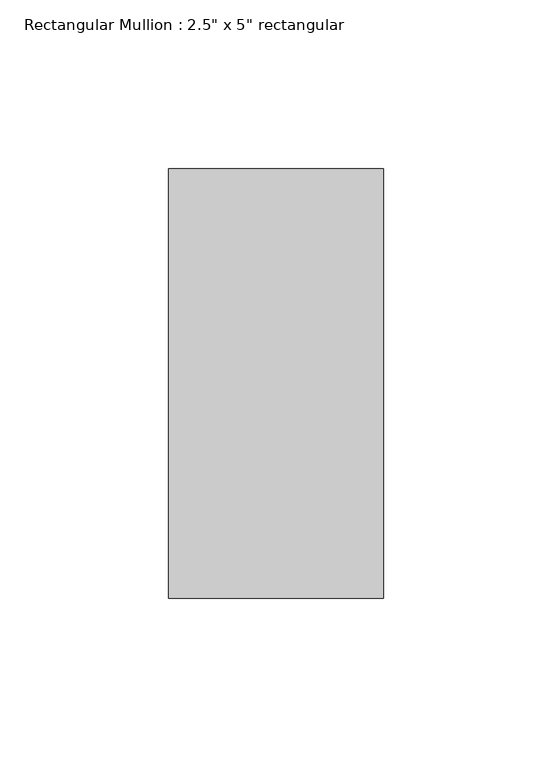
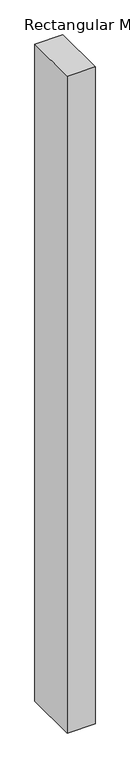
"""IFC4 building model written with IfcOpenShell, lengths in millimetres: member geometry."""

from ifc_helpers import new_model, si_unit, frame, origin, place, context, project, spatial, polyline, outline, extrude, source, transform, mapped, element, save


def member_ed31d27a(model_context):
    return source(origin(), model_context, "Body", "SweptSolid", [
        extrude(outline(polyline([(31.75, 63.5), (31.75, -63.5), (-31.75, -63.5), (-31.75, 63.5), (31.75, 63.5)])), frame((0.0, 0.0, -1579.2479304), z_axis=(0.0, 0.0, 1.0), x_axis=(1.0, 0.0, 0.0)), (0.0, 0.0, 1.0), 1579.2479304),
    ])


if __name__ == "__main__":
    model = new_model("IFC4")
    model_context = context("Model", 3, world=origin())
    ifc_project = project(units=[si_unit("LENGTHUNIT", "METRE", prefix="MILLI")], contexts=[model_context])
    site = spatial("IfcSite", under=ifc_project)
    building = spatial("IfcBuilding", under=site)
    placement = place(None, origin())
    member_shape = member_ed31d27a(model_context)
    element("IfcMember", 1, ObjectType="Rectangular Mullion : 2.5\" x 5\" rectangular", at=placement, inside=building, context=model_context, shape_type="MappedRepresentation", body=[
        mapped(member_shape, transform((0.0, 0.0, 0.0), x_axis=(1.0, 0.0, 0.0), y_axis=(0.0, 1.0, 0.0), z_axis=(0.0, 0.0, 1.0))),
    ])
    save(model, "model.ifc")

# Revit data of these elements
# Type "Rectangular Mullion : 2.5\" x 5\" rectangular"
#   built-in parameter 1007304 = 0.416667 (stored number, unit not read)
#   built-in parameter 1007301 = 0.104167 (stored number, unit not read)
#   built-in parameter 1007300 = 0.104167 (stored number, unit not read)
# Element 1 (IfcMember, "Rectangular Mullion : 2.5\" x 5\" rectangular")
#   Materials on its faces: "Aluminum"
# Materials
#   "Aluminum": class "Metal", colour RGB 247 247 247, transparency 0, Description = "Aluminum 6061", Cost = 0
